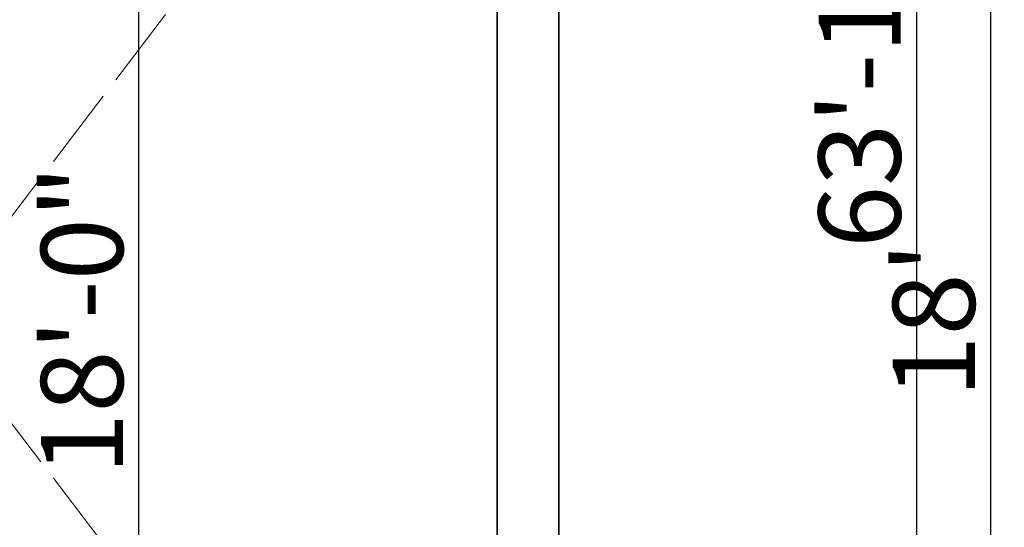
# Model space of a CAD drawing. Units: inches. Extents: x 2083 to 3317, y 1141 to 2115.
# Tile 253 of 256: x 3048 to 3192, y 1564 to 1639. Entities that reach past the tile are written whole.
import ezdxf

# ---------------------------------------------------------------- set-up
doc = ezdxf.new("R2010")
doc.units = ezdxf.units.IN
doc.linetypes.add('ACAD_ISO02W100', pattern=[15, 12, -3])
for name, color, linetype, lineweight in [('A-ANNO-DIMS', 2, 'Continuous', 18), ('A-FLOR-OPEN', 8, 'ACAD_ISO02W100', 13), ('A-WALL', 7, 'Continuous', 35)]:
    doc.layers.add(name, color=color, linetype=linetype, lineweight=lineweight)
doc.layers.add('A-WALL-PATT', color=251, linetype='Continuous', lineweight=13, true_color=0x636466)
doc.styles.get("Standard").update_dxf_attribs({"font": 'arial.ttf'})
doc.dimstyles.new('ISO-25', dxfattribs={"dimtxt": 12, "dimasz": 12, "dimexe": 1.25, "dimexo": 0.625, "dimtad": 1, "dimlunit": 3, "dimtxsty": 'Standard', "dimcen": 2.5, "dimadec": 0, "dimazin": 0, "dimtfac": 1, "dimtmove": 0, "dimatfit": 3, "dimfxl": 1, "dimarcsym": 0})

# ---------------------------------------------------------------- blocks, each defined once
blk = doc.blocks.new('*D8')
at = {"layer": 'A-ANNO-DIMS', "color": 0, "lineweight": -2, "transparency": 16777216}
for p, q in [((3127.58, 1702.76), (3191.32, 1702.76)), ((3190.07, 1690.76), (3190.07, 1498.76)), ((3127.58, 1486.76), (3191.32, 1486.76))]:
    blk.add_line(p, q, dxfattribs=at)
at = {"layer": 'A-ANNO-DIMS', "color": 0, "transparency": 16777216}
for points in [[(3188.07, 1690.76), (3192.07, 1690.76), (3190.07, 1702.76)], [(3188.07, 1498.76), (3192.07, 1498.76), (3190.07, 1486.76)]]:
    blk.add_solid(points, dxfattribs=at)
at = {"layer": 'Defpoints', "color": 0, "transparency": 16777216}
for p in [(3126.96, 1702.76), (3126.96, 1486.76), (3190.07, 1486.76)]:
    blk.add_point(p, dxfattribs=at)
at = {"layer": 'A-ANNO-DIMS', "color": 0, "transparency": 16777216, "insert": (3183.32, 1594.76), "char_height": 12, "attachment_point": 5, "rotation": 90}
blk.add_mtext("18'", dxfattribs=at)
blk = doc.blocks.new('*D35')
at = {"layer": 'A-ANNO-DIMS', "color": 0, "lineweight": -2, "transparency": 16777216}
for p, q in [((3127.58, 2020.76), (3180.56, 2020.76)), ((3179.31, 1275.26), (3179.31, 2008.76)), ((3127.58, 1263.26), (3180.56, 1263.26))]:
    blk.add_line(p, q, dxfattribs=at)
at = {"layer": 'A-ANNO-DIMS', "color": 0, "transparency": 16777216}
for points in [[(3177.31, 2008.76), (3181.31, 2008.76), (3179.31, 2020.76)], [(3177.31, 1275.26), (3181.31, 1275.26), (3179.31, 1263.26)]]:
    blk.add_solid(points, dxfattribs=at)
at = {"layer": 'Defpoints', "color": 0, "transparency": 16777216}
for p in [(3126.96, 2020.76), (3179.31, 2020.76), (3126.96, 1263.26)]:
    blk.add_point(p, dxfattribs=at)
at = {"layer": 'A-ANNO-DIMS', "color": 0, "transparency": 16777216, "insert": (3172.48, 1642.01), "char_height": 12, "attachment_point": 5, "rotation": 90}
blk.add_mtext('63\'-1 1/2"', dxfattribs=at)
blk = doc.blocks.new('*D65')
at = {"layer": 'A-ANNO-DIMS', "color": 0, "lineweight": -2, "transparency": 16777216}
for p, q in [((3117.33, 1702.76), (3064.36, 1702.76)), ((3065.61, 1498.76), (3065.61, 1690.76)), ((3117.33, 1486.76), (3064.36, 1486.76))]:
    blk.add_line(p, q, dxfattribs=at)
at = {"layer": 'A-ANNO-DIMS', "color": 0, "transparency": 16777216}
for points in [[(3063.61, 1690.76), (3067.61, 1690.76), (3065.61, 1702.76)], [(3063.61, 1498.76), (3067.61, 1498.76), (3065.61, 1486.76)]]:
    blk.add_solid(points, dxfattribs=at)
at = {"layer": 'Defpoints', "color": 0, "transparency": 16777216}
for p in [(3065.61, 1702.76), (3117.96, 1702.76), (3117.96, 1486.76)]:
    blk.add_point(p, dxfattribs=at)
at = {"layer": 'A-ANNO-DIMS', "color": 0, "transparency": 16777216, "insert": (3058.86, 1594.76), "char_height": 12, "attachment_point": 5, "rotation": 90}
blk.add_mtext('18\'-0"', dxfattribs=at)

msp = doc.modelspace()

# ---------------------------------------------------------------- hatches: boundary and pattern name
at = {"layer": 'A-WALL-PATT'}
h = msp.add_hatch(color=256, dxfattribs=at)
h.dxf.hatch_style = 1
h.paths.add_polyline_path([(3126.96, 2020.761), (2748.96, 2020.761), (2604.96, 2020.761), (2226.96, 2020.761), (2226.96, 1702.761), (2466.96, 1702.761), (2466.96, 1582.761), (2418.96, 1582.761), (2418.96, 1477.761), (2226.96, 1477.761), (2226.96, 1263.261), (2544.96, 1263.261), (2544.96, 1411.761), (2604.96, 1411.761), (2685.96, 1411.761), (2685.96, 1420.761), (2604.96, 1420.761), (2604.96, 1573.761), (2604.96, 1702.761), (2604.96, 2011.761), (2748.96, 2011.761), (2748.96, 1702.761), (2862.96, 1702.761), (2862.96, 1621.761), (2871.96, 1621.761), (2871.96, 1702.761), (2883.96, 1702.761), (2883.96, 1706.939, -0.0264593), (2883.96, 1711.761), (2757.96, 1711.761), (2757.96, 1807.761), (2787.96, 1807.761), (2787.96, 1812.261), (2757.96, 1812.261), (2757.96, 2011.761), (2877.96, 2011.761), (2877.96, 1812.261), (2847.96, 1812.261), (2847.96, 1807.761), (2889.836, 1807.761), (2889.836, 1812.261), (2882.46, 1812.261), (2882.46, 2011.761), (3117.96, 2011.761), (3117.96, 1812.261), (2937.836, 1812.261), (2937.836, 1807.761), (2995.71, 1807.761), (2995.71, 1796.118), (3000.21, 1796.118), (3000.21, 1807.761), (3117.96, 1807.761), (3117.96, 1711.761), (3000.21, 1711.761), (3000.21, 1760.118), (2998.573, 1760.118, -0.020711), (2995.71, 1760.118), (2995.71, 1711.761), (2931.96, 1711.761), (2931.96, 1702.761), (3126.96, 1702.761)])
h.paths.add_polyline_path([(2471.46, 2011.761), (2471.46, 1810.011), (2462.717, 1810.011), (2462.717, 1805.511), (2505.96, 1805.511), (2505.96, 1810.011), (2475.96, 1810.011), (2475.96, 2011.761), (2595.96, 2011.761), (2595.96, 1810.011), (2565.96, 1810.011), (2565.96, 1805.511), (2595.96, 1805.511), (2595.96, 1711.761), (2235.96, 1711.761), (2235.96, 1805.511), (2353.71, 1805.511), (2353.71, 1796.054), (2358.21, 1796.054), (2358.21, 1805.511), (2414.717, 1805.511), (2414.717, 1810.011), (2235.96, 1810.011), (2235.96, 2011.761)], flags=16)
h.paths.add_polyline_path([(2270.205, 1994.61), (2270.205, 1970.61), (2246.205, 1970.61), (2246.205, 1994.61)], flags=0)
edge = h.paths.add_edge_path(flags=0)
edge.add_ellipse((2332.027, 1899.798), major_axis=(-3.043, 3.043), ratio=0.1682525, start_angle=-161.33217, end_angle=-156.30711, ccw=False)
edge.add_ellipse((2333.082, 1898.744), major_axis=(-1.055, 1.055), ratio=0.4535321, start_angle=-123.37102, end_angle=-94.15911)
edge = h.paths.add_edge_path(flags=0)
edge.add_ellipse((2332.027, 1968.876), major_axis=(3.043, 3.043), ratio=0.1682525, start_angle=18.66783, end_angle=23.69289)
edge.add_spline(control_points=[(2332.926, 1970.691), (2332.227, 1970.336), (2330.894, 1969.659), (2328.413, 1970.932), (2327.204, 1967.749), (2324.71, 1969.956), (2322.533, 1967.012), (2320.013, 1971.296), (2317.68, 1968.158), (2316.041, 1967.102), (2315.427, 1966.81)], knot_values=[0, 0, 0, 0, 2.2670587, 4.3245589, 6.6855835, 8.8786411, 11.121502, 14.300359, 17.7552837, 19.732645, 19.732645, 19.732645, 19.732645], degree=3, periodic=0)
edge.add_ellipse((2332.027, 1968.876), major_axis=(3.043, 3.043), ratio=0.1682525, start_angle=18.66783, end_angle=23.69289, ccw=False)
edge.add_ellipse((2333.082, 1969.931), major_axis=(1.055, 1.055), ratio=0.4535321, start_angle=56.62898, end_angle=85.84089, ccw=False)
edge = h.paths.add_edge_path(flags=0)
edge.add_spline(control_points=[(2296.428, 1967.988), (2293.628, 1965.336), (2287.704, 1959.727), (2299.744, 1949.996), (2294.533, 1935.669), (2290.573, 1920.604), (2293.394, 1909.974), (2296.185, 1904.967)], knot_values=[0.0991853, 0.0991853, 0.0991853, 0.0991853, 0.3453009, 0.6198217, 0.9826526, 1.3860932, 1.8105546, 1.8105546, 1.8105546, 1.8105546], degree=3, periodic=0)
edge.add_spline(control_points=[(2296.185, 1904.967), (2297.384, 1902.619), (2298.001, 1901.949), (2298.553, 1901.468)], knot_values=[0.0062457, 0.0062457, 0.0062457, 0.0062457, 0.0554759, 0.0554759, 0.0554759, 0.0554759], degree=3, periodic=0)
edge.add_spline(control_points=[(2298.553, 1901.468), (2297.259, 1900.923), (2295.225, 1900.232), (2293.06, 1900.614), (2292.101, 1900.788), (2292.09, 1900.791)], knot_values=[0.3128349, 0.3128349, 0.3128349, 0.3128349, 0.4017797, 0.4749867, 0.4759027, 0.4759027, 0.4759027, 0.4759027], degree=3, periodic=0)
edge.add_arc((2292.794, 1904.664), 3.937, 215.4209, 259.69818, ccw=False)
edge.add_spline(control_points=[(2289.585, 1902.382), (2289.477, 1902.535), (2289.368, 1902.688), (2289.261, 1902.841)], knot_values=[0.1028719, 0.1028719, 0.1028719, 0.1028719, 0.1168958, 0.1168958, 0.1168958, 0.1168958], degree=3, periodic=0)
edge.add_spline(control_points=[(2289.261, 1902.841), (2288.687, 1902.55), (2287.64, 1902.02), (2285.881, 1901.874), (2283.853, 1901.504), (2281.72, 1899.711), (2278.467, 1899.493), (2276.157, 1901.883), (2272.259, 1899.804), (2267.778, 1901.843), (2262.244, 1900.184), (2257.415, 1901.782), (2254.318, 1900.726), (2253.178, 1900.337)], knot_values=[0, 0, 0, 0, 1.9079767, 3.4771759, 5.261074, 7.9728515, 11.6802485, 13.7179214, 16.9395917, 22.789562, 27.5025027, 33.5952153, 37.1456181, 37.1456181, 37.1456181, 37.1456181], degree=3, periodic=0)
edge.add_line((2253.178, 1900.337), (2250.244, 1902.841))
edge.add_line((2250.244, 1902.841), (2250.244, 1965.833))
edge.add_line((2250.244, 1965.833), (2253.178, 1968.337))
edge.add_spline(control_points=[(2253.178, 1968.337), (2254.318, 1967.948), (2257.415, 1966.892), (2262.244, 1968.49), (2267.778, 1966.831), (2271.527, 1968.537), (2273.876, 1967.828), (2274.207, 1967.728)], knot_values=[0, 0, 0, 0, 0.0901802, 0.2449351, 0.3646438, 0.5132331, 0.5378548, 0.5378548, 0.5378548, 0.5378548], degree=3, periodic=0)
edge.add_arc((2274.353, 1963.793), 3.937, 72.05113, 92.12795, ccw=False)
edge.add_arc((2281.297, 1985.23), 18.596, 252.05113, 288.56572)
edge.add_arc((2292.317, 1956.029), 12.646, 71.02679, 113.77822, ccw=False)
edge = h.paths.add_edge_path(flags=0)
edge.add_spline(control_points=[(2274.899, 1951.856), (2275.066, 1951.617), (2275.233, 1951.377), (2275.398, 1951.136)], knot_values=[1.4099157, 1.4099157, 1.4099157, 1.4099157, 1.4315903, 1.4315903, 1.4315903, 1.4315903], degree=3, periodic=0)
edge.add_spline(control_points=[(2275.398, 1951.136), (2275.792, 1950.562), (2276.179, 1949.984), (2276.546, 1949.397)], knot_values=[1.3582378, 1.3582378, 1.3582378, 1.3582378, 1.4099157, 1.4099157, 1.4099157, 1.4099157], degree=3, periodic=0)
edge.add_line((2276.546, 1949.397), (2277.437, 1947.862))
edge.add_spline(control_points=[(2277.437, 1947.862), (2276.304, 1945.673), (2274.64, 1942.427), (2274.632, 1938.094), (2272.799, 1930.852), (2274.356, 1943.897), (2275.948, 1947.923), (2276.546, 1949.397)], knot_values=[0.0056315, 0.0056315, 0.0056315, 0.0056315, 0.1860139, 0.2660015, 0.3570872, 0.5963902, 0.7397317, 0.7397317, 0.7397317, 0.7397317], degree=3, periodic=0)
edge.add_spline(control_points=[(2276.546, 1949.397), (2276.179, 1949.984), (2275.792, 1950.562), (2275.398, 1951.136)], knot_values=[1.3582378, 1.3582378, 1.3582378, 1.3582378, 1.4099157, 1.4099157, 1.4099157, 1.4099157], degree=3, periodic=0)
edge.add_spline(control_points=[(2275.398, 1951.136), (2274.943, 1950.08), (2274.208, 1948.025), (2273.935, 1944.851), (2272.469, 1937.627), (2273.466, 1945.696), (2274.701, 1951.059), (2274.899, 1951.856)], knot_values=[0.1043639, 0.1043639, 0.1043639, 0.1043639, 0.1896363, 0.2696239, 0.3607096, 0.6000126, 0.6446217, 0.6446217, 0.6446217, 0.6446217], degree=3, periodic=0)
h.paths.add_polyline_path([(2269.168, 1963.128, -0.3575267), (2268.171, 1960.976, -0.0925607), (2268.171, 1939.436, -0.3575267), (2269.168, 1937.285, -0.3575267), (2267.016, 1938.282, -0.1647847), (2254.686, 1938.282, -0.3575267), (2252.534, 1937.285, -0.3575267), (2253.531, 1939.436, -0.0925607), (2253.531, 1960.976, -0.3575267), (2252.534, 1963.128, -0.3575267), (2254.686, 1962.131, -0.1647847), (2267.016, 1962.131, -0.3575267)], flags=0)
h.paths.add_polyline_path([(2248.874, 1967.802), (2248.874, 1957.028), (2249.458, 1957.028), (2249.458, 1911.647), (2248.874, 1911.647), (2248.874, 1900.873), (2246.512, 1900.873, 0.1973271), (2244.15, 1902.457), (2244.15, 1966.218, 0.1973271), (2246.512, 1967.802)], flags=0)
h.paths.add_polyline_path([(2269.168, 1931.389, -0.3575267), (2268.171, 1929.238, -0.0925607), (2268.171, 1907.698, -0.3575267), (2269.168, 1905.547, -0.3575267), (2267.016, 1906.544, -0.1647847), (2254.686, 1906.544, -0.3575267), (2252.534, 1905.547, -0.3575267), (2253.531, 1907.698, -0.0925607), (2253.531, 1929.238, -0.3575267), (2252.534, 1931.389, -0.3575267), (2254.686, 1930.392, -0.1647847), (2267.016, 1930.392, -0.3575267)], flags=0)
edge = h.paths.add_edge_path(flags=0)
edge.add_spline(control_points=[(2276.197, 1906.724), (2276.168, 1909.029), (2276.114, 1913.372), (2270.598, 1924.925), (2273.905, 1919.013), (2275.922, 1916.262), (2275.475, 1912.402), (2277.258, 1910.381), (2276.696, 1908.225), (2276.646, 1906.813), (2276.618, 1906.008)], knot_values=[0, 0, 0, 0, 8.6102597, 16.2212739, 18.8430575, 23.8048978, 27.4408283, 29.3561016, 31.2034776, 33.6506866, 33.6506866, 33.6506866, 33.6506866], degree=3, periodic=0)
edge.add_spline(control_points=[(2276.618, 1906.008), (2276.623, 1905.624), (2276.498, 1904.629), (2275.442, 1903.855), (2274.937, 1903.08), (2274.859, 1902.841)], knot_values=[0.1564884, 0.1564884, 0.1564884, 0.1564884, 0.1843975, 0.2313765, 0.2505985, 0.2505985, 0.2505985, 0.2505985], degree=3, periodic=0)
edge.add_line((2274.859, 1902.841), (2276.506, 1902.841))
edge.add_spline(control_points=[(2276.506, 1902.841), (2276.788, 1903.085), (2277.665, 1904.125), (2278.25, 1904.341), (2277.654, 1908.527), (2278.156, 1906.228), (2278.1, 1905.286), (2278.847, 1904.069), (2277.857, 1903.415), (2277.874, 1902.991), (2277.904, 1902.841)], knot_values=[0.0595743, 0.0595743, 0.0595743, 0.0595743, 0.0807529, 0.1037415, 0.1697201, 0.1760361, 0.2071372, 0.2404744, 0.2623409, 0.2736605, 0.2736605, 0.2736605, 0.2736605], degree=3, periodic=0)
edge.add_line((2277.904, 1902.841), (2280.03, 1902.841))
edge.add_spline(control_points=[(2280.03, 1902.841), (2279.888, 1903.088), (2279.499, 1903.982), (2280.152, 1905.939), (2278.104, 1909.658), (2279.762, 1907.185), (2280.328, 1904.875), (2280.485, 1903.49), (2281.463, 1903.249), (2281.758, 1902.936), (2281.834, 1902.841)], knot_values=[0.013856, 0.013856, 0.013856, 0.013856, 0.0348738, 0.0888667, 0.1078792, 0.1267378, 0.158714, 0.1937575, 0.2174868, 0.2267221, 0.2267221, 0.2267221, 0.2267221], degree=3, periodic=0)
edge.add_spline(control_points=[(2281.834, 1902.841), (2281.788, 1902.827), (2281.647, 1902.783), (2281.396, 1902.859), (2281.088, 1902.985), (2280.721, 1903.061), (2280.333, 1903.026), (2280.125, 1902.899), (2280.03, 1902.841)], knot_values=[0, 0, 0, 0, 0.1441304, 0.435517, 0.7492759, 1.1530457, 1.5483707, 1.878348, 1.878348, 1.878348, 1.878348], degree=3, periodic=0)
edge.add_line((2280.03, 1902.841), (2277.904, 1902.841))
edge.add_spline(control_points=[(2277.904, 1902.841), (2277.893, 1902.796), (2277.865, 1902.68), (2277.607, 1902.687), (2277.274, 1902.801), (2276.838, 1902.62), (2276.584, 1902.789), (2276.506, 1902.841)], knot_values=[0, 0, 0, 0, 0.1271885, 0.3261988, 0.6280094, 1.2435704, 1.5153306, 1.5153306, 1.5153306, 1.5153306], degree=3, periodic=0)
edge.add_line((2276.506, 1902.841), (2274.859, 1902.841))
edge.add_spline(control_points=[(2274.859, 1902.841), (2274.814, 1902.899), (2274.725, 1903.013), (2274.493, 1903.119), (2274.244, 1902.961), (2273.937, 1903.185), (2273.614, 1902.983), (2273.408, 1902.883), (2273.322, 1902.841)], knot_values=[0, 0, 0, 0, 0.2184302, 0.4369566, 0.6879766, 0.9903786, 1.3983955, 1.6918498, 1.6918498, 1.6918498, 1.6918498], degree=3, periodic=0)
edge.add_spline(control_points=[(2273.322, 1902.841), (2273.617, 1903.446), (2274.274, 1904.538), (2276.027, 1904.574), (2276.207, 1906.584), (2276.197, 1906.724)], knot_values=[0.0122268, 0.0122268, 0.0122268, 0.0122268, 0.0594721, 0.1062177, 0.134458, 0.134458, 0.134458, 0.134458], degree=3, periodic=0)
h.paths.add_polyline_path([(2270.776, 1897.79), (2270.776, 1873.79), (2246.776, 1873.79), (2246.776, 1897.79)], flags=0)
h.paths.add_polyline_path([(2353.71, 1760.005), (2353.71, 1760.054), (2358.21, 1760.054, -0.033729)], flags=0)
h.paths.add_polyline_path([(2321.819, 1737.529), (2341.995, 1737.529, -0.4142136), (2343.203, 1736.321), (2343.203, 1721.021, -0.4142136), (2341.995, 1719.813), (2321.819, 1719.813, -0.4142136), (2320.611, 1721.021), (2320.611, 1736.321, -0.4142136)], flags=0)
h.paths.add_polyline_path([(2324.235, 1736.321), (2339.579, 1736.321, -0.4142136), (2341.995, 1733.905), (2341.995, 1725.45, -0.4142136), (2339.579, 1723.034), (2333.681, 1723.034), (2333.845, 1722.045, -0.8706461), (2335.425, 1721.826, -0.767327), (2333.923, 1721.423), (2331.291, 1721.423, -0.767327), (2329.788, 1721.826, -0.8706461), (2331.368, 1722.045), (2331.533, 1723.034), (2324.235, 1723.034, -0.4142136), (2321.819, 1725.45), (2321.819, 1733.905, -0.4142136)], flags=0)
h.paths.add_polyline_path([(2570.484, 1928.615), (2589.684, 1928.615), (2590.169, 1928.615), (2590.169, 1904.993), (2570.484, 1904.993)], flags=0)
h.paths.add_polyline_path([(2574.447, 1927.264, -1), (2572.829, 1927.264, -1)], flags=0)
h.paths.add_polyline_path([(2573.09, 1926.941), (2573.925, 1927.776), (2574.148, 1927.553), (2573.313, 1926.718)], flags=0)
h.paths.add_polyline_path([(2578.779, 1919.73, -1), (2571.592, 1919.73, -1)], flags=0)
h.paths.add_polyline_path([(2578.385, 1919.73, -1), (2571.985, 1919.73, -1)], flags=0)
h.paths.add_polyline_path([(2331.596, 1729.476, -1), (2333.618, 1729.476, -1)], flags=0)
h.paths.add_polyline_path([(2578.034, 1927.264, -1), (2576.416, 1927.264, -1)], flags=0)
h.paths.add_polyline_path([(2576.689, 1927.531), (2576.912, 1927.754), (2577.747, 1926.919), (2577.524, 1926.696)], flags=0)
h.paths.add_polyline_path([(2578.139, 1909.86, -1), (2572.232, 1909.86, -1)], flags=0)
h.paths.add_polyline_path([(2577.745, 1909.86, -1), (2572.625, 1909.86, -1)], flags=0)
h.paths.add_polyline_path([(2583.798, 1927.264, -1), (2582.179, 1927.264, -1)], flags=0)
h.paths.add_polyline_path([(2582.719, 1927.754), (2583.554, 1926.919), (2583.331, 1926.696), (2582.496, 1927.531)], flags=0)
h.paths.add_polyline_path([(2582.496, 1927.531), (2582.719, 1927.754), (2583.554, 1926.919), (2583.331, 1926.696)], flags=0)
h.paths.add_polyline_path([(2587.739, 1920.53, -1), (2581.832, 1920.53, -1)], flags=0)
h.paths.add_polyline_path([(2587.345, 1920.53, -1), (2582.225, 1920.53, -1)], flags=0)
h.paths.add_polyline_path([(2587.385, 1927.264, -1), (2585.766, 1927.264, -1)], flags=0)
h.paths.add_polyline_path([(2586.082, 1926.98), (2586.917, 1927.815), (2587.14, 1927.593), (2586.305, 1926.758)], flags=0)
h.paths.add_polyline_path([(2588.379, 1910.66, -1), (2581.192, 1910.66, -1)], flags=0)
h.paths.add_polyline_path([(2587.985, 1910.66, -1), (2581.585, 1910.66, -1)], flags=0)
h.paths.add_polyline_path([(2417.168, 1729.478), (2437.344, 1729.478, -0.4142136), (2438.552, 1728.27), (2438.552, 1712.969, -0.4142136), (2437.344, 1711.761), (2417.168, 1711.761, -0.4142136), (2415.96, 1712.969), (2415.96, 1728.27, -0.4142136)], flags=0)
h.paths.add_polyline_path([(2419.584, 1728.27), (2434.928, 1728.27, -0.4142136), (2437.344, 1725.854), (2437.344, 1717.398, -0.4142136), (2434.928, 1714.983), (2429.029, 1714.983), (2429.194, 1713.994, -0.8706461), (2430.774, 1713.775, -0.767327), (2429.271, 1713.372), (2426.64, 1713.372, -0.767327), (2425.137, 1713.775, -0.8706461), (2426.717, 1713.994), (2426.882, 1714.983), (2419.584, 1714.983, -0.4142136), (2417.168, 1717.398), (2417.168, 1725.854, -0.4142136)], flags=0)
h.paths.add_polyline_path([(2419.584, 1728.27), (2434.928, 1728.27, -0.4142136), (2437.344, 1725.854), (2437.344, 1717.398, -0.4142136), (2434.928, 1714.983), (2429.029, 1714.983), (2428.358, 1719.009), (2427.553, 1719.009), (2426.882, 1714.983), (2419.584, 1714.983, -0.4142136), (2417.168, 1717.398), (2417.168, 1725.854, -0.4142136)], flags=0)
h.paths.add_polyline_path([(2426.944, 1721.425, -1), (2428.967, 1721.425, -1)], flags=0)
h.paths.add_polyline_path([(2475.96, 1702.761), (2595.96, 1702.761), (2595.96, 1582.761), (2475.96, 1582.761)], flags=16)
h.paths.add_polyline_path([(2427.96, 1573.761), (2595.96, 1573.761), (2595.96, 1468.761), (2595.96, 1420.761), (2384.46, 1420.761), (2384.46, 1468.761), (2427.96, 1468.761)], flags=16)
h.paths.add_polyline_path([(2379.96, 1468.761), (2379.96, 1420.761), (2235.96, 1420.761), (2235.96, 1468.761)], flags=16)
h.paths.add_polyline_path([(2317.816, 1466.696), (2337.992, 1466.696, -0.4142136), (2339.2, 1465.488), (2339.2, 1450.187, -0.4142136), (2337.992, 1448.979), (2317.816, 1448.979, -0.4142136), (2316.608, 1450.187), (2316.608, 1465.488, -0.4142136)], flags=0)
h.paths.add_polyline_path([(2320.232, 1465.488), (2335.576, 1465.488, -0.4142136), (2337.992, 1463.072), (2337.992, 1454.616, -0.4142136), (2335.576, 1452.2), (2329.677, 1452.2), (2329.842, 1451.212, -0.8706461), (2331.422, 1450.992, -0.767327), (2329.92, 1450.59), (2327.288, 1450.59, -0.767327), (2325.785, 1450.992, -0.8706461), (2327.365, 1451.212), (2327.53, 1452.2), (2320.232, 1452.2, -0.4142136), (2317.816, 1454.616), (2317.816, 1463.072, -0.4142136)], flags=0)
h.paths.add_polyline_path([(2320.232, 1465.488), (2335.576, 1465.488, -0.4142136), (2337.992, 1463.072), (2337.992, 1454.616, -0.4142136), (2335.576, 1452.2), (2329.677, 1452.2), (2329.006, 1456.227), (2328.201, 1456.227), (2327.53, 1452.2), (2320.232, 1452.2, -0.4142136), (2317.816, 1454.616), (2317.816, 1463.072, -0.4142136)], flags=0)
h.paths.add_polyline_path([(2327.593, 1458.643, -1), (2329.615, 1458.643, -1)], flags=0)
h.paths.add_polyline_path([(2244.412, 1433.34), (2241.921, 1433.34, -0.4142136), (2240.018, 1435.244), (2240.018, 1440.953, -0.4142105), (2241.921, 1442.856), (2244.412, 1442.856, -1.9764724)], flags=0)
h.paths.add_polyline_path([(2245.357, 1434.398, -0.4142136), (2245.357, 1441.799, -2.1440985)], flags=0)
h.paths.add_polyline_path([(2535.96, 1416.261), (2535.96, 1272.261), (2235.96, 1272.261), (2235.96, 1416.261)], flags=16)
h.paths.add_polyline_path([(2260.12, 1384.293), (2260.12, 1362.039), (2237.865, 1362.039), (2237.865, 1384.293)], flags=0)
edge = h.paths.add_edge_path(flags=0)
edge.add_line((2318.252, 1362.093), (2318.146, 1362.001))
edge.add_ellipse((2317.445, 1360.431), major_axis=(2.822, 2.822), ratio=0.1682525, start_angle=18.66783, end_angle=20.94813, ccw=False)
edge.add_ellipse((2318.423, 1361.409), major_axis=(0.978, 0.978), ratio=0.4535321, start_angle=56.62898, end_angle=70.2262, ccw=False)
edge = h.paths.add_edge_path(flags=0)
edge.add_line((2319.107, 1295.571), (2319.015, 1295.677))
edge.add_ellipse((2317.445, 1296.378), major_axis=(-2.822, 2.822), ratio=0.1682525, start_angle=-161.33217, end_angle=-159.05187, ccw=False)
edge.add_ellipse((2318.423, 1295.4), major_axis=(-0.978, 0.978), ratio=0.4535321, start_angle=-123.37102, end_angle=-109.7738)
edge = h.paths.add_edge_path(flags=0)
edge.add_spline(control_points=[(2284.21, 1301.17), (2284.581, 1300.445), (2284.891, 1299.892), (2285.16, 1299.461)], knot_values=[0.0390658, 0.0390658, 0.0390658, 0.0390658, 0.0554759, 0.0554759, 0.0554759, 0.0554759], degree=3, periodic=0)
edge.add_line((2285.16, 1299.461), (2284.21, 1301.17))
edge = h.paths.add_edge_path(flags=0)
edge.add_line((2280.412, 1297.298), (2283.37, 1297.036))
edge.add_line((2283.37, 1297.036), (2286.406, 1297.926))
edge.add_spline(control_points=[(2286.406, 1297.926), (2285.305, 1297.463), (2284.345, 1297.129), (2283.37, 1297.036)], knot_values=[0.3943688, 0.3943688, 0.3943688, 0.3943688, 0.4759027, 0.4759027, 0.4759027, 0.4759027], degree=3, periodic=0)
edge.add_spline(control_points=[(2283.37, 1297.036), (2283.281, 1297.028), (2282.316, 1296.957), (2281.313, 1297.134), (2280.423, 1297.296), (2280.412, 1297.298)], knot_values=[0.3128349, 0.3128349, 0.3128349, 0.3128349, 0.3202458, 0.3934528, 0.3943688, 0.3943688, 0.3943688, 0.3943688], degree=3, periodic=0)
edge = h.paths.add_edge_path(flags=0)
edge.add_line((2284.436, 1359.607), (2280.446, 1355.328))
edge.add_line((2280.446, 1355.328), (2279.58, 1351.018))
edge.add_line((2279.58, 1351.018), (2282.413, 1346.58))
edge.add_spline(control_points=[(2282.413, 1346.58), (2283.153, 1345.589), (2284.253, 1344.029), (2284.801, 1342.387), (2284.935, 1341.806)], knot_values=[1.2400982, 1.2400982, 1.2400982, 1.2400982, 1.3328922, 1.3827123, 1.3827123, 1.3827123, 1.3827123], degree=3, periodic=0)
edge.add_spline(control_points=[(2284.935, 1341.806), (2285.319, 1340.141), (2285.233, 1338.409), (2284.91, 1336.654)], knot_values=[1.0974841, 1.0974841, 1.0974841, 1.0974841, 1.2400982, 1.2400982, 1.2400982, 1.2400982], degree=3, periodic=0)
edge.add_spline(control_points=[(2284.91, 1336.654), (2284.587, 1334.899), (2284.027, 1333.12), (2283.463, 1331.361)], knot_values=[0.9548699, 0.9548699, 0.9548699, 0.9548699, 1.0974841, 1.0974841, 1.0974841, 1.0974841], degree=3, periodic=0)
edge.add_line((2283.463, 1331.361), (2281.89, 1326.153))
edge.add_line((2281.89, 1326.153), (2280.756, 1321.056))
edge.add_line((2280.756, 1321.056), (2280.299, 1316.002))
edge.add_line((2280.299, 1316.002), (2280.716, 1310.95))
edge.add_line((2280.716, 1310.95), (2282.028, 1305.972))
edge.add_line((2282.028, 1305.972), (2284.21, 1301.17))
edge.add_spline(control_points=[(2284.21, 1301.17), (2283.341, 1302.73), (2282.612, 1304.336), (2282.028, 1305.972)], knot_values=[0.0991853, 0.0991853, 0.0991853, 0.0991853, 0.2417994, 0.2417994, 0.2417994, 0.2417994], degree=3, periodic=0)
edge.add_spline(control_points=[(2282.028, 1305.972), (2281.444, 1307.608), (2281.005, 1309.273), (2280.716, 1310.95)], knot_values=[0.2417994, 0.2417994, 0.2417994, 0.2417994, 0.3844135, 0.3844135, 0.3844135, 0.3844135], degree=3, periodic=0)
edge.add_spline(control_points=[(2280.716, 1310.95), (2280.433, 1312.588), (2280.289, 1314.277), (2280.299, 1315.962), (2280.299, 1316.002)], knot_values=[0.3844135, 0.3844135, 0.3844135, 0.3844135, 0.5236467, 0.5270276, 0.5270276, 0.5270276, 0.5270276], degree=3, periodic=0)
edge.add_spline(control_points=[(2280.299, 1316.002), (2280.312, 1317.687), (2280.478, 1319.368), (2280.756, 1321.056)], knot_values=[0.5270276, 0.5270276, 0.5270276, 0.5270276, 0.6696417, 0.6696417, 0.6696417, 0.6696417], degree=3, periodic=0)
edge.add_spline(control_points=[(2280.756, 1321.056), (2281.035, 1322.744), (2281.426, 1324.44), (2281.89, 1326.153)], knot_values=[0.6696417, 0.6696417, 0.6696417, 0.6696417, 0.8122558, 0.8122558, 0.8122558, 0.8122558], degree=3, periodic=0)
edge.add_spline(control_points=[(2281.89, 1326.153), (2282.264, 1327.533), (2282.788, 1329.262), (2283.353, 1331.018), (2283.463, 1331.361)], knot_values=[0.8122558, 0.8122558, 0.8122558, 0.8122558, 0.9270873, 0.9548699, 0.9548699, 0.9548699, 0.9548699], degree=3, periodic=0)
edge.add_line((2283.463, 1331.361), (2284.91, 1336.654))
edge.add_line((2284.91, 1336.654), (2284.935, 1341.806))
edge.add_line((2284.935, 1341.806), (2282.413, 1346.58))
edge.add_spline(control_points=[(2282.413, 1346.58), (2281.275, 1348.104), (2280.078, 1349.57), (2279.58, 1351.018)], knot_values=[1.3827123, 1.3827123, 1.3827123, 1.3827123, 1.5253264, 1.5253264, 1.5253264, 1.5253264], degree=3, periodic=0)
edge.add_spline(control_points=[(2279.58, 1351.018), (2279.443, 1351.415), (2279.136, 1352.857), (2279.735, 1354.29), (2280.446, 1355.328)], knot_values=[1.5253264, 1.5253264, 1.5253264, 1.5253264, 1.564439, 1.6679405, 1.6679405, 1.6679405, 1.6679405], degree=3, periodic=0)
edge.add_spline(control_points=[(2280.446, 1355.328), (2281.426, 1356.758), (2282.931, 1358.183), (2284.436, 1359.607)], knot_values=[1.6679405, 1.6679405, 1.6679405, 1.6679405, 1.8105546, 1.8105546, 1.8105546, 1.8105546], degree=3, periodic=0)
edge.add_arc((2280.623, 1348.518), 11.726, 71.02679, 113.77822)
edge.add_arc((2270.405, 1375.595), 17.244, 252.05113, 288.56572, ccw=False)
edge.add_arc((2263.966, 1355.718), 3.651, 72.05113, 92.12795)
edge.add_arc((2263.966, 1355.718), 3.651, 92.12795, 177.98513)
edge.add_spline(control_points=[(2260.318, 1355.846), (2260.26, 1354.221), (2260.551, 1350.187), (2262.999, 1346.766), (2264.473, 1344.649)], knot_values=[1.4315903, 1.4315903, 1.4315903, 1.4315903, 1.5641438, 1.7706953, 1.7706953, 1.7706953, 1.7706953], degree=3, periodic=0)
edge.add_line((2264.473, 1344.649), (2264.936, 1343.983))
edge.add_spline(control_points=[(2263.801, 1340.248), (2263.843, 1340.514), (2264.067, 1341.756), (2264.513, 1343.002), (2264.935, 1343.981)], knot_values=[0.5365702, 0.5365702, 0.5365702, 0.5365702, 0.5593494, 0.6446217, 0.6446217, 0.6446217, 0.6446217], degree=3, periodic=0)
edge.add_spline(control_points=[(2264.935, 1343.981), (2265.118, 1343.715), (2265.299, 1343.448), (2265.477, 1343.179)], knot_values=[1.3840767, 1.3840767, 1.3840767, 1.3840767, 1.4099157, 1.4099157, 1.4099157, 1.4099157], degree=3, periodic=0)
edge.add_spline(control_points=[(2265.477, 1343.179), (2265.655, 1342.911), (2265.829, 1342.641), (2265.999, 1342.369)], knot_values=[1.3582378, 1.3582378, 1.3582378, 1.3582378, 1.3840767, 1.3840767, 1.3840767, 1.3840767], degree=3, periodic=0)
edge.add_line((2265.999, 1342.369), (2266.826, 1340.946))
edge.add_spline(control_points=[(2266.826, 1340.946), (2268.894, 1337.09), (2271.398, 1325.843), (2270.516, 1310.569), (2275.919, 1301.861), (2277.79, 1299.199)], knot_values=[0.1168958, 0.1168958, 0.1168958, 0.1168958, 0.4729873, 1.0509689, 1.3137934, 1.3137934, 1.3137934, 1.3137934], degree=3, periodic=0)
edge.add_spline(control_points=[(2277.79, 1299.199), (2277.839, 1299.128), (2277.889, 1299.057), (2277.94, 1298.987)], knot_values=[0.1098839, 0.1098839, 0.1098839, 0.1098839, 0.1168958, 0.1168958, 0.1168958, 0.1168958], degree=3, periodic=0)
edge.add_line((2277.94, 1298.987), (2277.789, 1299.199))
edge.add_spline(control_points=[(2277.789, 1299.199), (2277.257, 1298.929), (2276.286, 1298.438), (2275.039, 1298.334), (2274.383, 1298.239), (2274.215, 1298.209)], knot_values=[33.1218702, 33.1218702, 33.1218702, 33.1218702, 35.0290557, 36.5982549, 37.1448269, 37.1448269, 37.1448269, 37.1448269], degree=3, periodic=0)
edge.add_line((2274.215, 1298.209), (2273.073, 1297.893))
edge.add_spline(control_points=[(2273.073, 1297.893), (2272.323, 1297.58), (2271.039, 1296.511), (2269.248, 1296.226), (2268.423, 1296.375)], knot_values=[26.5325843, 26.5325843, 26.5325843, 26.5325843, 29.198919, 31.8391012, 31.8391012, 31.8391012, 31.8391012], degree=3, periodic=0)
edge.add_line((2268.423, 1296.375), (2263.879, 1297.458))
edge.add_spline(control_points=[(2263.879, 1297.458), (2263.556, 1297.359), (2261.86, 1296.839), (2260.239, 1297.282), (2258.933, 1297.516)], knot_values=[15.9195506, 15.9195506, 15.9195506, 15.9195506, 16.9395917, 21.2260675, 21.2260675, 21.2260675, 21.2260675], degree=3, periodic=0)
edge.add_line((2258.933, 1297.516), (2254.055, 1297.329))
edge.add_spline(control_points=[(2254.055, 1297.329), (2253.756, 1297.296), (2252.114, 1297.165), (2250.462, 1297.544), (2249.13, 1297.668)], knot_values=[5.3065169, 5.3065169, 5.3065169, 5.3065169, 6.2764352, 10.6130337, 10.6130337, 10.6130337, 10.6130337], degree=3, periodic=0)
edge.add_line((2249.13, 1297.668), (2244.332, 1296.878))
edge.add_line((2244.332, 1296.878), (2241.611, 1299.199))
edge.add_line((2241.611, 1299.199), (2241.611, 1357.609))
edge.add_line((2241.611, 1357.609), (2244.332, 1359.931))
edge.add_line((2244.332, 1359.931), (2252.729, 1359.543))
edge.add_spline(control_points=[(2252.729, 1359.543), (2252.871, 1359.546), (2253.306, 1359.548), (2253.74, 1359.514), (2254.032, 1359.482)], knot_values=[0.233291, 0.233291, 0.233291, 0.233291, 0.2449351, 0.2689274, 0.2689274, 0.2689274, 0.2689274], degree=3, periodic=0)
edge.add_line((2254.032, 1359.482), (2259.587, 1359.416))
edge.add_spline(control_points=[(2259.587, 1359.416), (2260.677, 1359.629), (2262.073, 1359.897), (2263.524, 1359.459), (2263.83, 1359.366)], knot_values=[0.4225164, 0.4225164, 0.4225164, 0.4225164, 0.5132331, 0.5378548, 0.5378548, 0.5378548, 0.5378548], degree=3, periodic=0)
edge.add_arc((2263.966, 1355.718), 3.651, 72.05113, 92.12795, ccw=False)
edge.add_arc((2270.405, 1375.595), 17.244, 252.05113, 288.56572)
edge.add_arc((2280.623, 1348.518), 11.726, 71.02679, 113.77822, ccw=False)
h.paths.add_polyline_path([(2240.341, 1359.435), (2240.341, 1349.444), (2240.882, 1349.444), (2240.882, 1307.365), (2240.341, 1307.365), (2240.341, 1297.374), (2238.15, 1297.374, 0.1973271), (2235.96, 1298.843), (2235.96, 1357.966, 0.1973271), (2238.15, 1359.435)], flags=0)
h.paths.add_polyline_path([(2259.158, 1355.101, -0.3575267), (2258.233, 1353.106, -0.0925607), (2258.233, 1333.133, -0.3575267), (2259.158, 1331.138, -0.3575267), (2257.163, 1332.062, -0.1647847), (2245.729, 1332.062, -0.3575267), (2243.735, 1331.138, -0.3575267), (2244.659, 1333.133, -0.0925607), (2244.659, 1353.106, -0.3575267), (2243.735, 1355.101, -0.3575267), (2245.729, 1354.176, -0.1647847), (2257.163, 1354.176, -0.3575267)], flags=0)
edge = h.paths.add_edge_path(flags=0)
edge.add_line((2265.999, 1342.369), (2266.826, 1340.946))
edge.add_line((2266.826, 1340.946), (2265.308, 1337.814))
edge.add_line((2265.308, 1337.814), (2264.358, 1334.653))
edge.add_line((2264.358, 1334.653), (2264.262, 1333.8))
edge.add_spline(control_points=[(2264.262, 1333.8), (2264.208, 1333.187), (2264.162, 1332.366), (2264.007, 1331.414), (2263.969, 1331.202)], knot_values=[0.4644442, 0.4644442, 0.4644442, 0.4644442, 0.5166905, 0.5316081, 0.5316081, 0.5316081, 0.5316081], degree=3, periodic=0)
edge.add_spline(control_points=[(2263.969, 1331.202), (2263.775, 1330.119), (2263.424, 1328.791), (2263.257, 1328.531), (2263.234, 1328.515)], knot_values=[0.3726816, 0.3726816, 0.3726816, 0.3726816, 0.4488497, 0.4644442, 0.4644442, 0.4644442, 0.4644442], degree=3, periodic=0)
edge.add_spline(control_points=[(2263.234, 1328.515), (2263.096, 1328.42), (2263.131, 1329.301), (2263.275, 1330.616)], knot_values=[0.2809191, 0.2809191, 0.2809191, 0.2809191, 0.3726816, 0.3726816, 0.3726816, 0.3726816], degree=3, periodic=0)
edge.add_spline(control_points=[(2263.275, 1330.616), (2263.419, 1331.93), (2263.672, 1333.677), (2263.97, 1335.315)], knot_values=[0.1891566, 0.1891566, 0.1891566, 0.1891566, 0.2809191, 0.2809191, 0.2809191, 0.2809191], degree=3, periodic=0)
edge.add_spline(control_points=[(2263.97, 1335.315), (2264.1, 1336.032), (2264.419, 1337.622), (2264.755, 1338.864), (2264.947, 1339.491)], knot_values=[0.097394, 0.097394, 0.097394, 0.097394, 0.1375775, 0.1891566, 0.1891566, 0.1891566, 0.1891566], degree=3, periodic=0)
edge.add_spline(control_points=[(2264.947, 1339.491), (2265.29, 1340.606), (2265.644, 1341.494), (2265.999, 1342.369)], knot_values=[0.0056315, 0.0056315, 0.0056315, 0.0056315, 0.097394, 0.097394, 0.097394, 0.097394], degree=3, periodic=0)
h.paths.add_polyline_path([(2259.158, 1325.671, -0.3575267), (2258.233, 1323.676, -0.0925607), (2258.233, 1303.703, -0.3575267), (2259.158, 1301.708, -0.3575267), (2257.163, 1302.633, -0.1647847), (2245.729, 1302.633, -0.3575267), (2243.735, 1301.708, -0.3575267), (2244.659, 1303.703, -0.0925607), (2244.659, 1323.676, -0.3575267), (2243.735, 1325.671, -0.3575267), (2245.729, 1324.747, -0.1647847), (2257.163, 1324.747, -0.3575267)], flags=0)
edge = h.paths.add_edge_path(flags=0)
edge.add_spline(control_points=[(2261.709, 1317.311), (2261.679, 1317.418), (2261.762, 1317.389), (2262.491, 1316.09), (2262.962, 1315.301)], knot_values=[14.9558607, 14.9558607, 14.9558607, 14.9558607, 16.2212739, 18.6948259, 18.6948259, 18.6948259, 18.6948259], degree=3, periodic=0)
edge.add_spline(control_points=[(2262.962, 1315.301), (2262.99, 1315.254), (2263.702, 1314.067), (2264.349, 1313.127), (2264.73, 1312.164)], knot_values=[18.6948259, 18.6948259, 18.6948259, 18.6948259, 18.8430575, 22.433791, 22.433791, 22.433791, 22.433791], degree=3, periodic=0)
edge.add_spline(control_points=[(2264.73, 1312.164), (2264.876, 1311.796), (2265.177, 1310.77), (2265.143, 1309.559), (2265.248, 1308.824)], knot_values=[22.433791, 22.433791, 22.433791, 22.433791, 23.8048978, 26.1727562, 26.1727562, 26.1727562, 26.1727562], degree=3, periodic=0)
edge.add_line((2265.248, 1308.824), (2265.851, 1307.172))
edge.add_spline(control_points=[(2265.851, 1307.172), (2266.065, 1306.822), (2266.384, 1306.332), (2266.424, 1305.781), (2266.42, 1305.611)], knot_values=[28.0625624, 28.0625624, 28.0625624, 28.0625624, 29.3561016, 29.9117214, 29.9117214, 29.9117214, 29.9117214], degree=3, periodic=0)
edge.add_spline(control_points=[(2266.42, 1305.611), (2266.416, 1305.433), (2266.394, 1305.25), (2266.365, 1305.066)], knot_values=[29.9117214, 29.9117214, 29.9117214, 29.9117214, 30.4978371, 30.4978371, 30.4978371, 30.4978371], degree=3, periodic=0)
edge.add_line((2266.365, 1305.066), (2266.066, 1302.136))
edge.add_spline(control_points=[(2266.066, 1302.136), (2266.071, 1301.78), (2265.998, 1301.2), (2265.663, 1300.759), (2265.509, 1300.586)], knot_values=[0.1564884, 0.1564884, 0.1564884, 0.1564884, 0.1843975, 0.2035434, 0.2035434, 0.2035434, 0.2035434], degree=3, periodic=0)
edge.add_line((2265.509, 1300.586), (2264.435, 1299.199))
edge.add_line((2264.435, 1299.199), (2265.962, 1299.199))
edge.add_line((2265.962, 1299.199), (2267.336, 1301.175))
edge.add_line((2267.336, 1301.175), (2267.312, 1301.986))
edge.add_spline(control_points=[(2267.312, 1301.986), (2267.261, 1302.862), (2267.16, 1303.737), (2267.271, 1303.326)], knot_values=[0.1262286, 0.1262286, 0.1262286, 0.1262286, 0.1666174, 0.1666174, 0.1666174, 0.1666174], degree=3, periodic=0)
edge.add_spline(control_points=[(2267.271, 1303.326), (2267.28, 1303.294), (2267.31, 1303.175), (2267.373, 1302.884), (2267.406, 1302.683), (2267.418, 1302.601)], knot_values=[0.1666174, 0.1666174, 0.1666174, 0.1666174, 0.1697201, 0.1760361, 0.1807647, 0.1807647, 0.1807647, 0.1807647], degree=3, periodic=0)
edge.add_spline(control_points=[(2267.744, 1300.988), (2267.688, 1301.151), (2267.481, 1301.657), (2267.484, 1302.145), (2267.418, 1302.601)], knot_values=[0.1807647, 0.1807647, 0.1807647, 0.1807647, 0.1937665, 0.2201389, 0.2201389, 0.2201389, 0.2201389], degree=3, periodic=0)
edge.add_line((2267.418, 1302.601), (2267.744, 1300.988))
edge.add_spline(control_points=[(2267.744, 1300.988), (2267.832, 1300.732), (2267.932, 1300.31), (2267.555, 1299.975), (2267.429, 1299.829)], knot_values=[0.2201389, 0.2201389, 0.2201389, 0.2201389, 0.2404744, 0.2548903, 0.2548903, 0.2548903, 0.2548903], degree=3, periodic=0)
edge.add_line((2267.429, 1299.829), (2267.258, 1299.199))
edge.add_line((2267.258, 1299.199), (2269.23, 1299.199))
edge.add_spline(control_points=[(2269.23, 1299.199), (2269.099, 1299.429), (2268.843, 1300.016), (2269.012, 1300.916), (2268.947, 1301.661)], knot_values=[0.013856, 0.013856, 0.013856, 0.013856, 0.0348738, 0.0670726, 0.0670726, 0.0670726, 0.0670726], degree=3, periodic=0)
edge.add_line((2268.947, 1301.661), (2268.432, 1303.603))
edge.add_spline(control_points=[(2268.432, 1303.603), (2268.176, 1304.192), (2267.596, 1305.251), (2268.041, 1304.623), (2268.251, 1304.282)], knot_values=[0.0901547, 0.0901547, 0.0901547, 0.0901547, 0.1078792, 0.1202891, 0.1202891, 0.1202891, 0.1202891], degree=3, periodic=0)
edge.add_spline(control_points=[(2268.251, 1304.282), (2268.361, 1304.105), (2269.058, 1302.918), (2269.383, 1301.59), (2269.521, 1300.776), (2269.575, 1300.556)], knot_values=[0.1202891, 0.1202891, 0.1202891, 0.1202891, 0.1267378, 0.158714, 0.1735056, 0.1735056, 0.1735056, 0.1735056], degree=3, periodic=0)
edge.add_line((2269.575, 1300.556), (2270.686, 1299.421))
edge.add_spline(control_points=[(2270.686, 1299.421), (2270.767, 1299.357), (2270.838, 1299.281), (2270.903, 1299.199)], knot_values=[0.2181597, 0.2181597, 0.2181597, 0.2181597, 0.2267221, 0.2267221, 0.2267221, 0.2267221], degree=3, periodic=0)
edge.add_line((2270.937, 1299.193), (2270.903, 1299.199))
edge.add_spline(control_points=[(2270.903, 1299.199), (2270.86, 1299.186), (2270.73, 1299.146), (2270.496, 1299.216), (2270.272, 1299.308), (2270.121, 1299.348), (2270.063, 1299.36)], knot_values=[0.939174, 0.939174, 0.939174, 0.939174, 1.0833044, 1.3746911, 1.6884499, 1.878348, 1.878348, 1.878348, 1.878348], degree=3, periodic=0)
edge.add_line((2270.063, 1299.36), (2269.23, 1299.199))
edge.add_line((2269.23, 1299.199), (2267.258, 1299.199))
edge.add_spline(control_points=[(2267.258, 1299.199), (2267.248, 1299.157), (2267.223, 1299.05), (2266.984, 1299.057), (2266.809, 1299.116), (2266.677, 1299.109), (2266.637, 1299.105)], knot_values=[0.7576653, 0.7576653, 0.7576653, 0.7576653, 0.8848538, 1.0838641, 1.3856747, 1.5153306, 1.5153306, 1.5153306, 1.5153306], degree=3, periodic=0)
edge.add_spline(control_points=[(2266.637, 1299.105), (2266.485, 1299.089), (2266.236, 1299.017), (2266.035, 1299.151), (2265.962, 1299.199)], knot_values=[0, 0, 0, 0, 0.4859051, 0.7576653, 0.7576653, 0.7576653, 0.7576653], degree=3, periodic=0)
edge.add_line((2265.962, 1299.199), (2264.435, 1299.199))
edge.add_line((2264.435, 1299.199), (2263.858, 1299.367))
edge.add_spline(control_points=[(2263.858, 1299.367), (2263.819, 1299.371), (2263.78, 1299.386), (2263.74, 1299.402)], knot_values=[0.8459249, 0.8459249, 0.8459249, 0.8459249, 0.9786272, 0.9786272, 0.9786272, 0.9786272], degree=3, periodic=0)
edge.add_line((2263.722, 1299.396), (2263.01, 1299.199))
edge.add_spline(control_points=[(2263.01, 1299.199), (2263.246, 1299.683), (2263.506, 1300.128), (2263.873, 1300.408)], knot_values=[0.0122268, 0.0122268, 0.0122268, 0.0122268, 0.0529705, 0.0529705, 0.0529705, 0.0529705], degree=3, periodic=0)
edge.add_spline(control_points=[(2263.873, 1300.408), (2263.932, 1300.453), (2264.084, 1300.553), (2264.255, 1300.624), (2264.36, 1300.665)], knot_values=[0.0529705, 0.0529705, 0.0529705, 0.0529705, 0.0594721, 0.0690861, 0.0690861, 0.0690861, 0.0690861], degree=3, periodic=0)
edge.add_line((2264.36, 1300.665), (2265.142, 1301.078))
edge.add_line((2265.142, 1301.078), (2265.676, 1302.8))
edge.add_line((2265.676, 1302.8), (2265.541, 1305.704))
edge.add_line((2265.541, 1305.704), (2264.803, 1309.328))
edge.add_line((2264.803, 1309.328), (2263.041, 1314.092))
edge.add_spline(control_points=[(2263.041, 1314.092), (2262.384, 1315.671), (2261.796, 1316.998), (2261.709, 1317.311)], knot_values=[11.2168955, 11.2168955, 11.2168955, 11.2168955, 14.9558607, 14.9558607, 14.9558607, 14.9558607], degree=3, periodic=0)
h.paths.add_polyline_path([(2871.96, 1416.261), (2895.91, 1416.261), (2895.91, 1420.761), (2871.96, 1420.761), (2871.96, 1501.761), (2862.96, 1501.761), (2862.96, 1420.761), (2805.96, 1420.761), (2805.96, 1411.761), (2862.96, 1411.761), (2862.96, 1263.261), (3126.96, 1263.261), (3126.96, 1411.761), (3126.96, 1486.761), (2943.96, 1486.761), (2943.96, 1477.761), (2967.86, 1477.761), (2967.86, 1420.761), (2943.91, 1420.761), (2943.91, 1416.261), (3117.96, 1416.261), (3117.96, 1420.761), (2972.36, 1420.761), (2972.36, 1477.761), (3117.96, 1477.761), (3117.96, 1420.761), (3117.96, 1272.261), (2871.96, 1272.261)], flags=0)
h.paths.add_polyline_path([(2457.126, 1485.943), (2527.603, 1485.943), (2527.603, 1537.636), (2457.126, 1537.636)], flags=8)
h.paths.add_polyline_path([(2481.005, 1609.982), (2590.766, 1609.982), (2590.766, 1682.003), (2481.005, 1682.003)], flags=8)
h.paths.add_polyline_path([(2483.085, 1729.127), (2553.562, 1729.127), (2553.562, 1780.82), (2483.085, 1780.82)], flags=8)

# ---------------------------------------------------------------- linework, layer by layer
at = {"layer": 'A-FLOR-OPEN'}
for p, q in [((2952.96, 1486.761), (3117.96, 1702.761)), ((2952.96, 1702.761), (3117.96, 1486.761))]:
    msp.add_line(p, q, dxfattribs=at)
at = {"layer": 'A-WALL'}
for p, q in [((3117.96, 1702.761), (3117.96, 1486.761)), ((3126.96, 1702.761), (3126.96, 1411.761))]:
    msp.add_line(p, q, dxfattribs=at)

# ---------------------------------------------------------------- dimensions: what is measured, and where the dimension line sits
at = {"layer": 'A-ANNO-DIMS'}
for base, p1, p2, override, picture, middle in [((3179.31, 2020.761), (3126.96, 1263.261), (3126.96, 2020.761), {"dimdec": 1, "dimlfac": 1, "dimrnd": 0, "dimzin": 1, "dimdsep": 46, "dimlunit": 4, "dimfrac": 2}, '*D35', (3172.476, 1642.011)), ((3065.61, 1702.761), (3117.96, 1486.761), (3117.96, 1702.761), {"dimdec": 1, "dimlfac": 1, "dimrnd": 0, "dimzin": 1, "dimdsep": 46, "dimlunit": 4, "dimfrac": 2}, '*D65', (3058.858, 1594.761)), ((3190.068, 1486.761), (3126.96, 1702.761), (3126.96, 1486.761), {"dimclrd": 0, "dimclre": 0, "dimclrt": 0}, '*D8', (3183.316, 1594.761))]:
    dim = msp.add_linear_dim(base=base, p1=p1, p2=p2, angle=90, dimstyle='ISO-25', override=override, dxfattribs=at)
    dim.commit()
    dim.dimension.update_dxf_attribs({"geometry": picture, "text_midpoint": middle})

doc.saveas('drawing.dxf')
